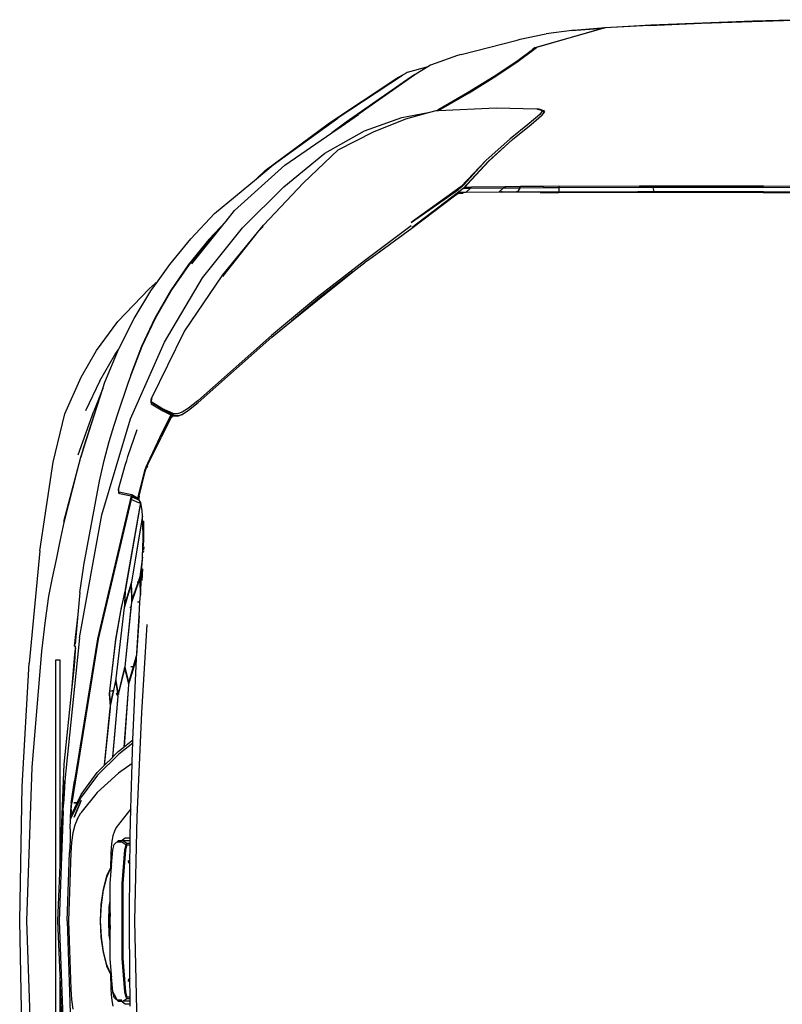
# Model space of a CAD drawing. Units: inches. Extents: x 22042254 to 25404563, y 17568978 to 17626777.
# Tile 3 of 45: x 22042254.0718 to 22042254.5426, y 17568978.1657 to 17568978.7735. Entities that reach past the tile are written whole.
import ezdxf

# ---------------------------------------------------------------- set-up
doc = ezdxf.new("R2010")
doc.units = ezdxf.units.IN
doc.header["$MEASUREMENT"] = 0
doc.layers.add('A-SITE-VEHI', color=8, linetype='Continuous', lineweight=18)
doc.layers.add('Edges', color=250, linetype='Continuous')

# ---------------------------------------------------------------- blocks, each defined once
blk = doc.blocks.new('Nissan Qashqai pl')
at = {"layer": 'Edges'}
for p, q in [((7.32157, 11.66208), (7.32157, 12.18208)), ((7.32607, 12.18208), (7.32607, 11.97794)), ((7.29801, 12.07497), (7.29279, 11.92208)), ((7.33017, 12.07853), (7.32607, 11.97794)), ((7.28835, 12.05625), (7.28572, 11.92208)), ((7.32507, 11.92208), (7.32911, 12.03155)), ((7.40018, 11.92208), (7.40245, 12.02601)), ((7.33294, 11.92208), (7.33653, 12.02372)), ((7.33733, 12.00038), (7.33865, 12.00996)), ((7.37751, 12.0015), (7.37864, 12.00699)), ((7.39589, 12.00706), (7.39588, 12.00508)), ((7.33667, 11.99003), (7.33733, 12.00038)), ((7.37683, 11.99537), (7.37751, 12.0015)), ((7.37985, 11.99831), (7.3787, 11.99283)), ((7.38081, 11.99933), (7.37985, 11.99831)), ((7.38074, 11.99908), (7.37985, 11.99831)), ((7.38002, 11.99534), (7.38305, 12.00106)), ((7.38074, 11.99908), (7.38081, 11.99933)), ((7.38104, 11.99933), (7.38074, 11.99908)), ((7.38081, 11.99933), (7.38402, 12.00208)), ((7.38104, 11.99933), (7.38081, 11.99933)), ((7.38305, 12.00106), (7.38104, 11.99933)), ((7.38659, 12.00106), (7.38305, 12.00106)), ((7.38402, 12.00208), (7.38696, 12.00208)), ((7.38683, 12.00198), (7.38659, 12.00106)), ((7.3875, 12.00106), (7.38659, 12.00106)), ((7.38696, 12.00208), (7.38683, 12.00198)), ((7.39094, 12.00508), (7.38696, 12.00208)), ((7.38696, 12.00208), (7.38847, 12.00208)), ((7.38847, 12.00208), (7.39254, 11.99933)), ((7.39551, 12.00208), (7.38847, 12.00208)), ((7.39041, 11.99283), (7.39156, 11.99831)), ((7.39564, 12.00508), (7.39094, 12.00508)), ((7.39288, 11.99808), (7.39173, 11.99259)), ((7.39254, 11.99933), (7.39582, 11.99933)), ((7.39254, 11.99933), (7.39288, 11.99808)), ((7.3958, 11.99808), (7.39288, 11.99808)), ((7.39551, 12.00208), (7.39584, 12.00183)), ((7.39588, 12.0049), (7.39564, 12.00508)), ((7.39588, 12.00508), (7.39564, 12.00508)), ((7.3958, 11.99808), (7.39564, 11.98012)), ((7.39582, 11.99933), (7.3958, 11.99808)), ((7.39584, 12.00183), (7.39582, 11.99933)), ((7.39588, 12.0049), (7.39584, 12.00183)), ((7.39588, 12.00508), (7.39588, 12.0049)), ((7.33429, 11.92208), (7.33667, 11.99003)), ((7.37614, 11.97511), (7.37648, 11.98901)), ((7.37648, 11.98901), (7.37683, 11.99537)), ((7.3787, 11.99283), (7.37743, 11.97775)), ((7.3787, 11.99283), (7.38002, 11.99534)), ((7.38759, 11.95948), (7.39041, 11.99283)), ((7.39173, 11.99259), (7.38892, 11.95935)), ((7.32607, 11.9764), (7.32607, 11.97794)), ((7.37614, 11.97511), (7.37686, 11.97673)), ((7.37686, 11.97673), (7.3771, 11.97702)), ((7.37713, 11.97709), (7.3771, 11.97702)), ((7.37743, 11.97775), (7.37713, 11.97709)), ((7.37713, 11.97709), (7.3774, 11.97738)), ((7.3774, 11.97738), (7.37727, 11.97594)), ((7.3774, 11.97738), (7.37743, 11.97775)), ((7.39385, 11.98229), (7.39564, 11.98012)), ((7.39563, 11.97885), (7.39385, 11.981)), ((7.39563, 11.97885), (7.3951, 11.92208)), ((7.39564, 11.98012), (7.39563, 11.97885)), ((7.32607, 11.9764), (7.3238, 11.92208)), ((7.37239, 11.9667), (7.37614, 11.97511)), ((7.37707, 11.97569), (7.37268, 11.96585)), ((7.37727, 11.97594), (7.37588, 11.95948)), ((7.37727, 11.97594), (7.37707, 11.97569)), ((7.36896, 11.95363), (7.37239, 11.9667)), ((7.37268, 11.96585), (7.36932, 11.95303)), ((7.37588, 11.95948), (7.37588, 11.94171)), ((7.38759, 11.88468), (7.38759, 11.95948)), ((7.38892, 11.95935), (7.38892, 11.88481)), ((7.36681, 11.93841), (7.36896, 11.95363)), ((7.36932, 11.95303), (7.3672, 11.9381)), ((7.36607, 11.92208), (7.36681, 11.93841)), ((7.3672, 11.9381), (7.36648, 11.92208)), ((7.37588, 11.94171), (7.37512, 11.93632)), ((7.37588, 11.94171), (7.37588, 11.93029)), ((7.37512, 11.93632), (7.37448, 11.92208)), ((7.37551, 11.92208), (7.37588, 11.93029)), ((7.37588, 11.93029), (7.37588, 11.91388)), ((7.28572, 11.92208), (7.28835, 11.78791)), ((7.29279, 11.92208), (7.29801, 11.76919)), ((7.3238, 11.92208), (7.32607, 11.86622)), ((7.32911, 11.81261), (7.32507, 11.92208)), ((7.33294, 11.92208), (7.33535, 11.85392)), ((7.33667, 11.85414), (7.33429, 11.92208)), ((7.36681, 11.90575), (7.36607, 11.92208)), ((7.36648, 11.92208), (7.3672, 11.90606)), ((7.37448, 11.92208), (7.37512, 11.90785)), ((7.37588, 11.91388), (7.37551, 11.92208)), ((7.3951, 11.92208), (7.39563, 11.86531)), ((7.40245, 11.81815), (7.40018, 11.92208)), ((7.37588, 11.91388), (7.37588, 11.90246)), ((7.36896, 11.89053), (7.36681, 11.90575)), ((7.3672, 11.90606), (7.36932, 11.89113)), ((7.37512, 11.90785), (7.37588, 11.90246)), ((7.37588, 11.90246), (7.37588, 11.88468)), ((7.37239, 11.87746), (7.36896, 11.89053)), ((7.36932, 11.89113), (7.37268, 11.87831)), ((7.37588, 11.88468), (7.37727, 11.86822)), ((7.39041, 11.85133), (7.38759, 11.88468)), ((7.38892, 11.88481), (7.39173, 11.85157)), ((7.37614, 11.86905), (7.37239, 11.87746)), ((7.37268, 11.87831), (7.37707, 11.86848)), ((7.37648, 11.85515), (7.37614, 11.86905)), ((7.37686, 11.86743), (7.37614, 11.86905)), ((7.32607, 11.86622), (7.33017, 11.76563)), ((7.32607, 11.86622), (7.32607, 11.66208)), ((7.3771, 11.86714), (7.37686, 11.86743)), ((7.37707, 11.86848), (7.37727, 11.86822)), ((7.3771, 11.86714), (7.37713, 11.86707)), ((7.37713, 11.86707), (7.37743, 11.86641)), ((7.3774, 11.86678), (7.37713, 11.86707)), ((7.37727, 11.86822), (7.3774, 11.86678)), ((7.3774, 11.86678), (7.37743, 11.86641)), ((7.37743, 11.86641), (7.3787, 11.85133)), ((7.39385, 11.86316), (7.39563, 11.86531)), ((7.39564, 11.86404), (7.39385, 11.86187)), ((7.39563, 11.86531), (7.39564, 11.86404)), ((7.39564, 11.86404), (7.3958, 11.84608)), ((7.33608, 11.84164), (7.33535, 11.85392)), ((7.33733, 11.84378), (7.33667, 11.85414)), ((7.37683, 11.8488), (7.37648, 11.85515)), ((7.3787, 11.85133), (7.37985, 11.84585)), ((7.39156, 11.84585), (7.39041, 11.85133)), ((7.39173, 11.85157), (7.39288, 11.84608)), ((7.33619, 11.83012), (7.33608, 11.84164)), ((7.33865, 11.8342), (7.33733, 11.84378)), ((7.37751, 11.84267), (7.37683, 11.8488)), ((7.37864, 11.83717), (7.37751, 11.84267)), ((7.37985, 11.84585), (7.38081, 11.84483)), ((7.38081, 11.84483), (7.38074, 11.84508)), ((7.38081, 11.84483), (7.38104, 11.84483)), ((7.38402, 11.84208), (7.38081, 11.84483)), ((7.38305, 11.8431), (7.3875, 11.8431)), ((7.38696, 11.84208), (7.38402, 11.84208)), ((7.38696, 11.84208), (7.39094, 11.83908)), ((7.38847, 11.84208), (7.38696, 11.84208)), ((7.3875, 11.8431), (7.39156, 11.84585)), ((7.39254, 11.84483), (7.38847, 11.84208)), ((7.39551, 11.84208), (7.38847, 11.84208)), ((7.39288, 11.84608), (7.39254, 11.84483)), ((7.39582, 11.84483), (7.39254, 11.84483)), ((7.39288, 11.84608), (7.3958, 11.84608)), ((7.39584, 11.84233), (7.39551, 11.84208)), ((7.39564, 11.83908), (7.39587, 11.83925)), ((7.3958, 11.84608), (7.39582, 11.84483)), ((7.39582, 11.84483), (7.39584, 11.84233)), ((7.39584, 11.84233), (7.39587, 11.83925)), ((7.39587, 11.83925), (7.39587, 11.83908)), ((7.33619, 11.83012), (7.33653, 11.82044)), ((7.3407, 11.82658), (7.33865, 11.8342)), ((7.38014, 11.8327), (7.37864, 11.83717)), ((7.38184, 11.82907), (7.38014, 11.8327)), ((7.39094, 11.83908), (7.39564, 11.83908)), ((7.39564, 11.83908), (7.39587, 11.83908)), ((7.39587, 11.83908), (7.39589, 11.8371)), ((7.39589, 11.8371), (7.3966, 11.81032)), ((7.33615, 11.81939), (7.33653, 11.82044)), ((7.33672, 11.81955), (7.33615, 11.81939)), ((7.33653, 11.82044), (7.34711, 11.79873)), ((7.34316, 11.82104), (7.3407, 11.82658)), ((7.34316, 11.82104), (7.34679, 11.81424)), ((7.3966, 11.81032), (7.38184, 11.82907)), ((7.32911, 11.81261), (7.32941, 11.80569)), ((7.33645, 11.81201), (7.33615, 11.81939)), ((7.33691, 11.80472), (7.33645, 11.81201)), ((7.33686, 11.81546), (7.33737, 11.81653)), ((7.33691, 11.81132), (7.33686, 11.81546)), ((7.33686, 11.81546), (7.33805, 11.81508)), ((7.33691, 11.81132), (7.33767, 11.80437)), ((7.33737, 11.81653), (7.33805, 11.81508)), ((7.33805, 11.81508), (7.34299, 11.80448)), ((7.34013, 11.81856), (7.34308, 11.8112)), ((7.347, 11.80211), (7.34013, 11.81856)), ((7.34308, 11.8112), (7.347, 11.80211)), ((7.36303, 11.79404), (7.34679, 11.81424)), ((7.3966, 11.81032), (7.39782, 11.76508)), ((7.40723, 11.71423), (7.40245, 11.81815)), ((7.33008, 11.79493), (7.32941, 11.80569)), ((7.3295, 11.80119), (7.33087, 11.78224)), ((7.3295, 11.80119), (7.33008, 11.79493)), ((7.33691, 11.80472), (7.34048, 11.78254)), ((7.33771, 11.80416), (7.33767, 11.80437)), ((7.34104, 11.78371), (7.33771, 11.80416)), ((7.34299, 11.80448), (7.33961, 11.8043)), ((7.33961, 11.8043), (7.34314, 11.80416)), ((7.34299, 11.80448), (7.34314, 11.80416)), ((7.34314, 11.80416), (7.34693, 11.79606)), ((7.33087, 11.78224), (7.33008, 11.79493)), ((7.34693, 11.79606), (7.36309, 11.77403)), ((7.36331, 11.77672), (7.34711, 11.79873)), ((7.38423, 11.77487), (7.36303, 11.79404)), ((7.28835, 11.78791), (7.29513, 11.66508)), ((7.33168, 11.77242), (7.33087, 11.78224)), ((7.36347, 11.6409), (7.34048, 11.78254)), ((7.34263, 11.77348), (7.34104, 11.78371)), ((7.34554, 11.63996), (7.33168, 11.77242)), ((7.36397, 11.64129), (7.34263, 11.77348)), ((7.36309, 11.77403), (7.37008, 11.76708)), ((7.38449, 11.75584), (7.36331, 11.77672)), ((7.39782, 11.76508), (7.38423, 11.77487)), ((7.29801, 11.76919), (7.30777, 11.65317)), ((7.33017, 11.76563), (7.33778, 11.69209)), ((7.37589, 11.71006), (7.37008, 11.76708)), ((7.37008, 11.76708), (7.37036, 11.76681)), ((7.37036, 11.76681), (7.37608, 11.71004)), ((7.37036, 11.76681), (7.37826, 11.75896)), ((7.39782, 11.76508), (7.39816, 11.75211)), ((7.38357, 11.6983), (7.37826, 11.75896)), ((7.37826, 11.75896), (7.37876, 11.75846)), ((7.37876, 11.75846), (7.38403, 11.69824)), ((7.37876, 11.75846), (7.38409, 11.75317)), ((7.38409, 11.75317), (7.38964, 11.74878)), ((7.39848, 11.74482), (7.38449, 11.75584)), ((7.39816, 11.75211), (7.39848, 11.74482)), ((7.39414, 11.68653), (7.38964, 11.74878)), ((7.38964, 11.74878), (7.39027, 11.74828)), ((7.39027, 11.74828), (7.39449, 11.68648)), ((7.39027, 11.74828), (7.39862, 11.74167)), ((7.39848, 11.74482), (7.39862, 11.74167)), ((7.39862, 11.74167), (7.40182, 11.66777)), ((7.41241, 11.62655), (7.40723, 11.71423)), ((7.37498, 11.69572), (7.37596, 11.70814)), ((7.37623, 11.70617), (7.37575, 11.69593)), ((7.37596, 11.70814), (7.37589, 11.71006)), ((7.37608, 11.71004), (7.37634, 11.7081)), ((7.37623, 11.70617), (7.37642, 11.70614)), ((7.37634, 11.7081), (7.38127, 11.68424)), ((7.37642, 11.70614), (7.37916, 11.6924)), ((7.33778, 11.69209), (7.34072, 11.65629)), ((7.33778, 11.69209), (7.33996, 11.67104)), ((7.38128, 11.64204), (7.37498, 11.69572)), ((7.37575, 11.69593), (7.37562, 11.69326)), ((7.37916, 11.6924), (7.37562, 11.69326)), ((7.37562, 11.69326), (7.38154, 11.64126)), ((7.37568, 11.69592), (7.37575, 11.69593)), ((7.38118, 11.68226), (7.37916, 11.6924)), ((7.38174, 11.68442), (7.38322, 11.69486)), ((7.38379, 11.69443), (7.38202, 11.68226)), ((7.38243, 11.69547), (7.38357, 11.6983)), ((7.3835, 11.69733), (7.38243, 11.69547)), ((7.38336, 11.69586), (7.38243, 11.69547)), ((7.38243, 11.69547), (7.38322, 11.69486)), ((7.38324, 11.69498), (7.38243, 11.69547)), ((7.38322, 11.69486), (7.38379, 11.69443)), ((7.38324, 11.69498), (7.38336, 11.69586)), ((7.38377, 11.69466), (7.38324, 11.69498)), ((7.3837, 11.696), (7.38336, 11.69586)), ((7.3835, 11.69733), (7.38357, 11.6983)), ((7.38361, 11.69752), (7.3835, 11.69733)), ((7.38361, 11.69752), (7.38357, 11.6983)), ((7.38403, 11.69824), (7.38361, 11.69752)), ((7.38438, 11.69629), (7.3837, 11.696)), ((7.38377, 11.69466), (7.3837, 11.696)), ((7.38426, 11.69437), (7.38377, 11.69466)), ((7.38429, 11.69425), (7.38379, 11.69443)), ((7.38426, 11.69437), (7.38438, 11.69629)), ((7.38429, 11.69425), (7.38426, 11.69437)), ((7.38773, 11.68027), (7.38429, 11.69425)), ((7.38438, 11.69629), (7.39028, 11.67251)), ((7.38152, 11.68035), (7.38118, 11.68226)), ((7.38127, 11.68424), (7.38174, 11.68442)), ((7.3817, 11.68412), (7.38127, 11.68424)), ((7.3817, 11.68412), (7.38174, 11.68442)), ((7.38202, 11.68226), (7.38195, 11.68031)), ((7.39093, 11.67275), (7.39387, 11.6846)), ((7.39425, 11.68274), (7.39127, 11.6705)), ((7.39387, 11.6846), (7.39414, 11.68653)), ((7.39425, 11.68274), (7.39494, 11.68257)), ((7.39425, 11.68274), (7.39497, 11.68247)), ((7.39449, 11.68648), (7.39509, 11.68353)), ((7.39497, 11.68247), (7.39494, 11.68257)), ((7.39898, 11.66858), (7.39497, 11.68247)), ((7.39509, 11.68353), (7.40207, 11.66087)), ((7.38995, 11.60941), (7.38152, 11.68035)), ((7.38195, 11.68031), (7.39032, 11.60945)), ((7.38737, 11.68027), (7.38773, 11.68027)), ((7.39008, 11.67074), (7.38773, 11.68027)), ((7.39093, 11.67275), (7.39028, 11.67251)), ((7.39087, 11.67252), (7.39028, 11.67251)), ((7.39087, 11.67252), (7.39093, 11.67275)), ((7.3059, 11.55319), (7.29513, 11.66508)), ((7.33996, 11.67104), (7.34097, 11.65941)), ((7.39046, 11.66873), (7.39008, 11.67074)), ((7.3966, 11.6095), (7.39046, 11.66873)), ((7.39127, 11.6705), (7.39107, 11.66865)), ((7.39107, 11.66865), (7.39768, 11.60417)), ((7.39898, 11.66858), (7.39666, 11.66858)), ((7.4017, 11.65916), (7.39898, 11.66858)), ((7.40182, 11.66777), (7.40224, 11.66093)), ((7.30777, 11.65317), (7.31133, 11.62243)), ((7.32607, 11.66208), (7.32157, 11.66208)), ((7.34072, 11.65629), (7.34131, 11.65087)), ((7.34097, 11.65941), (7.34133, 11.65108)), ((7.40216, 11.65713), (7.4017, 11.65916)), ((7.40224, 11.66093), (7.40207, 11.66087)), ((7.40224, 11.66086), (7.40207, 11.66087)), ((7.40484, 11.618), (7.40216, 11.65713)), ((7.40224, 11.66093), (7.40224, 11.66086)), ((7.40224, 11.66086), (7.40484, 11.618)), ((7.34009, 11.64801), (7.34004, 11.64799)), ((7.3438, 11.61665), (7.34004, 11.64799)), ((7.34097, 11.64796), (7.34009, 11.64801)), ((7.34097, 11.64796), (7.34131, 11.65087)), ((7.34097, 11.64796), (7.34145, 11.64799)), ((7.34144, 11.64796), (7.34097, 11.64796)), ((7.3438, 11.61665), (7.34121, 11.64598)), ((7.34133, 11.65108), (7.34131, 11.65087)), ((7.34131, 11.65087), (7.34154, 11.6488)), ((7.34554, 11.63996), (7.36761, 11.51724)), ((7.39705, 11.49808), (7.36347, 11.6409)), ((7.39678, 11.50175), (7.36397, 11.64129)), ((7.3869, 11.60943), (7.38128, 11.64204)), ((7.38154, 11.64126), (7.38644, 11.61311)), ((7.31133, 11.62243), (7.31494, 11.59842)), ((7.34574, 11.59466), (7.3438, 11.61665)), ((7.40484, 11.618), (7.40567, 11.60418)), ((7.38644, 11.61311), (7.39089, 11.59332)), ((7.39116, 11.59143), (7.3869, 11.60943)), ((7.39012, 11.60735), (7.38995, 11.60941)), ((7.39099, 11.59348), (7.39012, 11.60735)), ((7.39032, 11.60945), (7.3908, 11.60755)), ((7.39058, 11.60552), (7.39095, 11.60545)), ((7.39058, 11.60552), (7.39098, 11.60538)), ((7.39058, 11.60552), (7.39141, 11.59144)), ((7.3908, 11.60755), (7.39654, 11.58812)), ((7.39098, 11.60538), (7.39095, 11.60545)), ((7.39668, 11.58624), (7.39098, 11.60538)), ((7.3966, 11.6095), (7.39566, 11.6095)), ((7.39715, 11.60416), (7.3966, 11.6095)), ((7.39722, 11.60211), (7.39715, 11.60416)), ((7.39768, 11.60417), (7.39823, 11.60225)), ((7.40567, 11.60418), (7.40319, 11.60418)), ((7.40567, 11.60418), (7.40611, 11.59696)), ((7.31494, 11.59842), (7.3186, 11.58002)), ((7.34574, 11.59466), (7.34938, 11.57004)), ((7.39684, 11.58823), (7.39722, 11.60211)), ((7.39774, 11.60029), (7.39733, 11.58621)), ((7.39774, 11.60029), (7.39827, 11.60018)), ((7.39774, 11.60029), (7.39831, 11.60008)), ((7.39823, 11.60225), (7.40485, 11.58292)), ((7.39831, 11.60008), (7.39827, 11.60018)), ((7.40376, 11.5843), (7.39831, 11.60008)), ((7.40533, 11.58312), (7.40611, 11.59688)), ((7.40611, 11.59688), (7.40611, 11.59696)), ((7.40611, 11.59688), (7.40642, 11.59185)), ((7.39099, 11.59348), (7.39089, 11.59332)), ((7.39101, 11.59337), (7.39089, 11.59332)), ((7.39156, 11.58943), (7.39116, 11.59143)), ((7.39141, 11.59144), (7.39169, 11.5895)), ((7.40622, 11.5053), (7.39156, 11.58943)), ((7.39169, 11.5895), (7.40648, 11.50498)), ((7.39684, 11.58823), (7.39654, 11.58812)), ((7.39714, 11.58424), (7.39668, 11.58624)), ((7.39684, 11.58823), (7.39731, 11.58844)), ((7.40828, 11.51835), (7.39714, 11.58424)), ((7.39733, 11.58621), (7.39747, 11.58427)), ((7.39747, 11.58427), (7.40836, 11.51976)), ((7.40376, 11.5843), (7.40279, 11.5843)), ((7.40488, 11.58107), (7.40376, 11.5843)), ((7.40642, 11.59185), (7.40597, 11.58338)), ((7.40642, 11.59185), (7.40687, 11.58436)), ((7.40687, 11.58436), (7.40791, 11.56437)), ((7.3186, 11.58002), (7.32232, 11.56164)), ((7.40533, 11.58312), (7.40485, 11.58292)), ((7.40532, 11.58299), (7.40485, 11.58292)), ((7.40539, 11.57906), (7.40488, 11.58107)), ((7.40597, 11.58327), (7.40532, 11.58299)), ((7.40532, 11.58299), (7.40533, 11.58312)), ((7.40597, 11.58338), (7.40533, 11.58312)), ((7.40814, 11.55935), (7.40539, 11.57906)), ((7.40597, 11.58327), (7.40585, 11.58097)), ((7.40585, 11.58097), (7.40588, 11.57905)), ((7.40588, 11.57905), (7.40791, 11.56437)), ((7.40597, 11.58338), (7.40597, 11.58327)), ((7.40813, 11.57111), (7.40752, 11.58276)), ((7.34938, 11.57004), (7.3497, 11.56742)), ((7.34938, 11.57004), (7.34978, 11.56736)), ((7.3497, 11.56742), (7.36534, 11.48377)), ((7.40791, 11.56437), (7.40811, 11.56038)), ((7.40791, 11.56437), (7.40812, 11.56285)), ((7.32232, 11.56164), (7.3261, 11.54328)), ((7.40811, 11.56038), (7.40814, 11.55935)), ((7.40814, 11.55935), (7.40871, 11.54047)), ((7.40926, 11.55458), (7.40949, 11.55292)), ((7.3059, 11.55319), (7.31925, 11.46451)), ((7.40923, 11.54161), (7.40902, 11.54853)), ((7.4096, 11.54898), (7.40916, 11.55209)), ((7.3261, 11.54328), (7.32996, 11.52493)), ((7.40871, 11.54047), (7.40865, 11.52464)), ((7.40921, 11.52579), (7.40923, 11.54161)), ((7.40908, 11.52353), (7.40921, 11.52579)), ((7.3297, 11.52373), (7.34671, 11.45961)), ((7.32996, 11.52493), (7.34671, 11.45961)), ((7.36761, 11.51724), (7.39627, 11.42146)), ((7.40828, 11.51835), (7.40795, 11.51289)), ((7.40836, 11.51976), (7.40828, 11.51835)), ((7.40865, 11.52464), (7.40836, 11.51976)), ((7.40795, 11.51289), (7.4066, 11.50521)), ((7.38529, 11.49584), (7.38412, 11.49562)), ((7.38437, 11.49158), (7.38412, 11.49562)), ((7.39764, 11.49714), (7.38458, 11.49463)), ((7.38529, 11.49584), (7.38458, 11.49463)), ((7.38529, 11.49584), (7.39705, 11.49808)), ((7.40464, 11.5053), (7.39678, 11.50175)), ((7.39804, 11.49925), (7.39678, 11.50175)), ((7.39705, 11.49808), (7.39833, 11.49833)), ((7.40264, 11.50022), (7.39764, 11.49714)), ((7.39804, 11.49925), (7.40478, 11.50242)), ((7.4012, 11.50009), (7.39804, 11.49925)), ((7.39833, 11.49833), (7.4012, 11.50009)), ((7.4012, 11.50009), (7.40335, 11.50141)), ((7.40299, 11.50047), (7.40264, 11.50022)), ((7.40299, 11.50047), (7.40276, 11.50042)), ((7.40326, 11.50066), (7.40299, 11.50047)), ((7.40417, 11.50199), (7.40326, 11.50066)), ((7.4033, 11.50053), (7.40326, 11.50066)), ((7.40335, 11.50054), (7.4033, 11.50053)), ((7.41007, 11.47333), (7.4033, 11.50053)), ((7.40335, 11.50141), (7.40417, 11.50199)), ((7.40425, 11.50164), (7.40405, 11.50122)), ((7.40431, 11.5014), (7.40405, 11.50122)), ((7.40405, 11.50122), (7.41077, 11.47382)), ((7.40417, 11.50199), (7.40443, 11.50199)), ((7.40425, 11.50164), (7.40417, 11.50199)), ((7.40443, 11.50199), (7.40425, 11.50164)), ((7.40431, 11.5014), (7.40425, 11.50164)), ((7.40461, 11.50161), (7.40431, 11.5014)), ((7.40447, 11.50076), (7.40431, 11.5014)), ((7.40456, 11.50227), (7.40443, 11.50199)), ((7.40443, 11.50199), (7.40463, 11.50199)), ((7.4048, 11.50082), (7.40447, 11.50076)), ((7.40502, 11.49854), (7.40447, 11.50076)), ((7.40456, 11.50227), (7.40478, 11.50242)), ((7.40497, 11.50227), (7.40456, 11.50227)), ((7.40456, 11.50227), (7.40463, 11.50199)), ((7.40469, 11.50176), (7.40461, 11.50161)), ((7.40463, 11.50199), (7.40469, 11.50176)), ((7.40463, 11.50199), (7.40482, 11.50199)), ((7.40622, 11.5053), (7.40464, 11.5053)), ((7.40482, 11.50199), (7.40469, 11.50176)), ((7.40478, 11.50242), (7.40523, 11.50274)), ((7.40515, 11.5026), (7.40478, 11.50242)), ((7.40497, 11.50227), (7.40482, 11.50199)), ((7.40515, 11.5026), (7.40497, 11.50227)), ((7.40523, 11.50274), (7.40515, 11.5026)), ((7.40632, 11.5047), (7.40523, 11.50274)), ((7.40632, 11.5047), (7.40622, 11.5053)), ((7.40648, 11.50498), (7.40632, 11.5047)), ((7.4066, 11.50521), (7.40648, 11.50498)), ((7.38458, 11.49463), (7.38437, 11.49158)), ((7.38437, 11.49158), (7.39136, 11.46669)), ((7.36534, 11.48377), (7.36995, 11.46286)), ((7.39136, 11.46669), (7.39248, 11.46286)), ((7.41147, 11.46951), (7.41007, 11.47333)), ((7.41077, 11.47382), (7.41219, 11.47)), ((7.41315, 11.46587), (7.41147, 11.46951)), ((7.41219, 11.47), (7.41393, 11.46637)), ((7.41256, 11.46999), (7.41248, 11.47021)), ((7.41324, 11.46853), (7.41256, 11.46999)), ((7.41393, 11.46637), (7.42672, 11.44006)), ((7.31925, 11.46451), (7.3309, 11.41659)), ((7.34401, 11.45722), (7.35959, 11.41392)), ((7.34891, 11.45171), (7.34671, 11.45961)), ((7.34671, 11.45961), (7.36864, 11.39135)), ((7.36995, 11.46286), (7.375, 11.44419)), ((7.39248, 11.46286), (7.39374, 11.45905)), ((7.39374, 11.45905), (7.40289, 11.43211)), ((7.42553, 11.43981), (7.41315, 11.46587)), ((7.34891, 11.45171), (7.36864, 11.39135)), ((7.375, 11.44419), (7.37986, 11.42777)), ((7.42553, 11.43981), (7.43673, 11.41738)), ((7.43787, 11.41791), (7.42672, 11.44006)), ((7.37986, 11.42777), (7.38454, 11.41358)), ((7.39627, 11.42146), (7.43015, 11.3449)), ((7.43587, 11.41698), (7.43673, 11.41738)), ((7.43832, 11.417), (7.43673, 11.41738)), ((7.43751, 11.42004), (7.43844, 11.41817)), ((7.43787, 11.41791), (7.43844, 11.41817)), ((7.4389, 11.41727), (7.43787, 11.41791)), ((7.43832, 11.417), (7.43787, 11.41791)), ((7.4389, 11.41727), (7.43832, 11.417)), ((7.43844, 11.41817), (7.43873, 11.41831)), ((7.43873, 11.41831), (7.44298, 11.41881)), ((7.4389, 11.41727), (7.44004, 11.41781)), ((7.44418, 11.41831), (7.44004, 11.41781)), ((7.44298, 11.41881), (7.44771, 11.41717)), ((7.44771, 11.41717), (7.44418, 11.41831)), ((7.44771, 11.41717), (7.45415, 11.41285)), ((7.3309, 11.41659), (7.34698, 11.37976)), ((7.36552, 11.38372), (7.3514, 11.41334)), ((7.36864, 11.39135), (7.35959, 11.41392)), ((7.38454, 11.41358), (7.39247, 11.38995)), ((7.42821, 11.41133), (7.41689, 11.40438)), ((7.41697, 11.40649), (7.42833, 11.41346)), ((7.42961, 11.41292), (7.4183, 11.40596)), ((7.43873, 11.41619), (7.42821, 11.41133)), ((7.42833, 11.41346), (7.43587, 11.41698)), ((7.42961, 11.41292), (7.43832, 11.417)), ((7.44309, 11.41655), (7.43873, 11.41619)), ((7.44789, 11.41487), (7.44309, 11.41655)), ((7.4541, 11.41081), (7.44789, 11.41487)), ((7.46355, 11.40337), (7.4541, 11.41081)), ((7.45415, 11.41285), (7.46382, 11.40513)), ((7.41665, 11.40488), (7.41697, 11.40649)), ((7.41716, 11.40469), (7.41665, 11.40488)), ((7.41687, 11.40359), (7.41665, 11.40488)), ((7.41687, 11.40359), (7.41686, 11.40296)), ((7.41686, 11.40296), (7.41723, 11.40107)), ((7.41689, 11.40438), (7.41687, 11.40359)), ((7.41717, 11.40184), (7.41687, 11.40359)), ((7.41716, 11.40469), (7.41689, 11.40438)), ((7.4183, 11.40596), (7.41716, 11.40469)), ((7.41744, 11.4013), (7.41717, 11.40184)), ((7.41723, 11.40107), (7.44978, 11.33488)), ((7.41744, 11.4013), (7.41747, 11.40124)), ((7.53689, 11.33848), (7.46355, 11.40337)), ((7.46382, 11.40513), (7.53708, 11.33997)), ((7.36864, 11.39135), (7.37074, 11.38491)), ((7.39247, 11.38995), (7.39379, 11.3859)), ((7.34698, 11.37976), (7.36237, 11.35349)), ((7.36552, 11.38372), (7.38053, 11.35758)), ((7.37074, 11.38491), (7.38426, 11.35219)), ((7.39379, 11.3859), (7.39513, 11.38217)), ((7.39513, 11.38217), (7.39648, 11.37869)), ((7.39621, 11.37814), (7.39648, 11.37869)), ((7.40715, 11.34933), (7.39621, 11.37814)), ((7.39648, 11.37869), (7.39687, 11.3777)), ((7.39687, 11.3777), (7.40781, 11.34902)), ((7.36237, 11.35349), (7.38367, 11.32447)), ((7.38053, 11.35758), (7.38426, 11.35219)), ((7.38426, 11.35219), (7.38446, 11.35171)), ((7.38446, 11.35171), (7.39973, 11.32146)), ((7.42053, 11.32124), (7.40715, 11.34933)), ((7.40781, 11.34902), (7.42115, 11.32101)), ((7.43015, 11.3449), (7.46788, 11.28072)), ((7.58274, 11.30006), (7.53689, 11.33848)), ((7.53708, 11.33997), (7.55684, 11.32404)), ((7.44978, 11.33488), (7.48836, 11.27781)), ((7.38367, 11.32447), (7.41469, 11.29179)), ((7.39973, 11.32146), (7.41661, 11.29389)), ((7.43626, 11.29398), (7.42053, 11.32124)), ((7.42115, 11.32101), (7.4369, 11.29377)), ((7.58398, 11.30127), (7.55684, 11.32404)), ((7.55684, 11.32404), (7.58288, 11.30303)), ((7.6296, 11.2639), (7.58274, 11.30006)), ((7.58288, 11.30303), (7.61803, 11.27504)), ((7.61803, 11.27504), (7.58398, 11.30127)), ((7.41469, 11.29179), (7.42386, 11.28371)), ((7.41661, 11.29389), (7.42386, 11.28371)), ((7.45423, 11.26769), (7.43626, 11.29398)), ((7.4369, 11.29377), (7.45491, 11.26748)), ((7.42386, 11.28371), (7.4354, 11.26752)), ((7.46788, 11.28072), (7.50805, 11.2311)), ((7.48817, 11.27966), (7.52431, 11.23409)), ((7.48836, 11.27781), (7.52891, 11.22832)), ((7.61803, 11.27504), (7.63007, 11.26544)), ((7.4354, 11.26752), (7.45654, 11.24186)), ((7.47438, 11.24268), (7.45423, 11.26769)), ((7.45491, 11.26748), (7.47504, 11.24255)), ((7.45735, 11.26699), (7.48846, 11.22834)), ((7.67598, 11.22893), (7.6296, 11.2639)), ((7.63007, 11.26544), (7.63056, 11.26506)), ((7.63056, 11.26506), (7.63059, 11.26504)), ((7.63059, 11.26504), (7.6373, 11.26013)), ((7.6373, 11.26013), (7.67691, 11.23122)), ((7.45654, 11.24186), (7.48015, 11.2168)), ((7.49177, 11.22424), (7.47438, 11.24268)), ((7.47504, 11.24255), (7.47703, 11.24044)), ((7.47703, 11.24044), (7.47653, 11.24106)), ((7.47703, 11.24053), (7.47751, 11.23993)), ((7.47838, 11.23878), (7.47703, 11.24044)), ((7.47703, 11.24044), (7.47751, 11.23993)), ((7.47751, 11.23993), (7.47871, 11.23847)), ((7.47751, 11.23993), (7.47869, 11.23868)), ((7.47869, 11.23868), (7.47824, 11.23925)), ((7.4795, 11.2377), (7.47869, 11.23868)), ((7.47869, 11.23868), (7.48846, 11.22834)), ((7.50805, 11.2311), (7.5492, 11.19016)), ((7.52431, 11.23409), (7.52857, 11.22958)), ((7.67691, 11.23122), (7.71943, 11.19922)), ((7.72318, 11.19554), (7.67713, 11.2307)), ((7.48846, 11.22834), (7.49177, 11.22424)), ((7.49177, 11.22424), (7.50008, 11.21391)), ((7.52891, 11.22832), (7.56866, 11.18624)), ((7.72614, 11.18985), (7.67617, 11.22557)), ((7.67617, 11.22557), (7.72327, 11.1928)), ((7.48015, 11.2168), (7.52174, 11.18228)), ((7.50008, 11.21391), (7.55011, 11.16843)), ((7.71943, 11.19922), (7.72318, 11.19658)), ((7.72318, 11.19658), (7.72785, 11.19647)), ((7.72807, 11.19181), (7.72318, 11.19554)), ((7.72318, 11.19554), (7.72455, 11.19553)), ((7.72667, 11.19023), (7.72327, 11.1928)), ((7.72467, 11.19542), (7.72455, 11.19553)), ((7.72455, 11.19553), (7.72942, 11.19548)), ((7.72807, 11.19181), (7.72986, 11.19044)), ((7.73491, 11.19175), (7.72807, 11.19181)), ((7.75301, 11.16475), (7.72807, 11.19181)), ((7.72942, 11.19548), (7.73096, 11.19549)), ((7.73096, 11.19549), (7.73491, 11.19175)), ((7.73096, 11.19549), (7.76399, 11.19528)), ((7.76799, 11.19147), (7.73491, 11.19175)), ((7.76399, 11.19528), (7.7636, 11.19566)), ((7.76799, 11.19147), (7.76399, 11.19528)), ((7.76399, 11.19528), (7.76622, 11.19527)), ((7.76586, 11.19567), (7.76622, 11.19527)), ((7.76622, 11.19527), (7.76683, 11.19458)), ((7.76622, 11.19527), (7.78115, 11.19519)), ((7.76925, 11.19146), (7.76799, 11.19147)), ((7.78439, 11.19133), (7.76925, 11.19146)), ((7.78115, 11.19519), (7.78091, 11.19575)), ((7.7814, 11.19458), (7.78115, 11.19519)), ((7.78115, 11.19519), (7.78224, 11.19518)), ((7.78224, 11.19518), (7.78192, 11.19576)), ((7.78224, 11.19518), (7.80566, 11.19505)), ((7.78439, 11.19133), (7.78224, 11.19518)), ((7.80777, 11.19113), (7.78439, 11.19133)), ((7.80482, 11.19588), (7.82329, 11.1958)), ((7.80566, 11.19505), (7.82329, 11.19498)), ((7.82329, 11.19498), (7.82329, 11.1958)), ((7.82329, 11.1958), (7.90142, 11.19549)), ((7.82329, 11.19498), (7.90204, 11.19468)), ((7.82329, 11.19107), (7.82329, 11.19498)), ((7.90142, 11.19549), (7.91849, 11.19552)), ((7.90204, 11.19468), (7.91833, 11.1947)), ((7.91833, 11.1947), (7.9176, 11.19075)), ((7.91849, 11.19552), (7.91833, 11.1947)), ((7.91833, 11.1947), (8.02749, 11.19482)), ((7.91849, 11.19552), (8.02732, 11.19568)), ((8.02732, 11.19568), (8.17527, 11.1963)), ((8.02749, 11.19482), (8.08756, 11.19507)), ((7.53043, 11.17373), (7.52174, 11.18228)), ((7.52174, 11.18228), (7.53868, 11.16822)), ((7.5492, 11.19016), (7.58999, 11.1565)), ((7.56866, 11.18624), (7.60319, 11.15334)), ((7.72614, 11.18985), (7.75074, 11.16383)), ((7.72856, 11.18809), (7.72667, 11.19023)), ((7.75074, 11.16383), (7.72856, 11.18809)), ((7.72986, 11.19044), (7.73238, 11.18764)), ((7.72986, 11.19044), (7.73635, 11.19039)), ((7.73238, 11.18764), (7.75388, 11.16419)), ((7.7363, 11.19044), (7.73635, 11.19039)), ((7.76942, 11.19011), (7.73635, 11.19039)), ((7.76942, 11.19011), (7.76874, 11.19075)), ((7.7707, 11.1901), (7.76942, 11.19011)), ((7.78514, 11.18998), (7.7707, 11.1901)), ((7.78462, 11.19091), (7.78514, 11.18998)), ((7.80829, 11.18979), (7.78514, 11.18998)), ((7.82329, 11.19107), (7.80777, 11.19113)), ((7.90396, 11.18944), (7.80829, 11.18979)), ((7.82329, 11.18994), (7.82329, 11.19107)), ((7.90357, 11.19074), (7.82329, 11.19107)), ((7.9176, 11.19075), (7.90357, 11.19074)), ((8.02759, 11.18962), (7.90396, 11.18944)), ((8.0275, 11.19086), (7.9176, 11.19075)), ((8.08729, 11.1911), (8.0275, 11.19086)), ((8.17534, 11.1903), (8.02759, 11.18962)), ((7.53043, 11.17373), (7.59458, 11.12619)), ((7.53868, 11.16822), (7.60312, 11.12171)), ((7.55011, 11.16843), (7.59689, 11.13645)), ((7.77477, 11.14231), (7.75074, 11.16383)), ((7.75301, 11.16475), (7.77724, 11.14311)), ((7.75388, 11.16419), (7.77724, 11.14311)), ((7.58999, 11.1565), (7.62951, 11.13442)), ((7.60319, 11.15334), (7.63858, 11.13525)), ((7.79381, 11.1271), (7.77477, 11.14231)), ((7.77724, 11.14311), (7.79586, 11.12808)), ((7.61132, 11.12557), (7.59689, 11.13645)), ((7.59689, 11.13645), (7.6021, 11.13289)), ((7.6021, 11.13289), (7.61183, 11.12554)), ((7.6021, 11.13289), (7.62368, 11.11814)), ((7.62951, 11.13442), (7.66697, 11.12116)), ((7.63858, 11.13525), (7.67084, 11.12249)), ((7.59458, 11.12619), (7.66077, 11.0825)), ((7.67585, 11.08087), (7.61132, 11.12557)), ((7.61183, 11.12554), (7.67993, 11.07831)), ((7.80447, 11.11791), (7.79381, 11.1271)), ((7.79586, 11.12808), (7.80619, 11.11916)), ((7.66763, 11.07907), (7.60245, 11.12206)), ((7.66697, 11.12116), (7.69488, 11.11584)), ((7.67084, 11.12249), (7.69488, 11.11584)), ((7.69488, 11.11584), (7.70101, 11.11415)), ((7.70101, 11.11415), (7.70235, 11.11408)), ((7.70382, 11.11316), (7.70235, 11.11408)), ((7.70235, 11.11408), (7.70343, 11.11403)), ((7.70343, 11.11403), (7.70559, 11.11279)), ((7.70343, 11.11403), (7.76082, 11.11124)), ((7.73247, 11.09659), (7.70382, 11.11316)), ((7.70559, 11.11279), (7.73411, 11.09632)), ((7.80216, 11.1126), (7.80721, 11.11412)), ((7.80956, 11.11476), (7.80372, 11.11265)), ((7.80721, 11.11412), (7.80447, 11.11791)), ((7.80867, 11.11585), (7.80619, 11.11916)), ((7.80619, 11.11916), (7.80665, 11.11877)), ((7.80665, 11.11877), (7.80956, 11.11476)), ((7.80721, 11.11412), (7.80867, 11.11585)), ((7.76082, 11.11124), (7.80143, 11.11238)), ((7.80143, 11.11238), (7.80216, 11.1126)), ((7.80372, 11.11265), (7.80216, 11.1126)), ((7.75906, 11.08002), (7.73247, 11.09659)), ((7.73411, 11.09632), (7.76061, 11.0798)), ((7.67122, 11.0767), (7.66077, 11.0825)), ((7.67207, 11.07622), (7.67122, 11.0767)), ((7.6926, 11.07047), (7.67207, 11.07622)), ((7.67933, 11.07844), (7.67585, 11.08087)), ((7.68018, 11.07816), (7.67933, 11.07844)), ((7.68018, 11.07816), (7.67993, 11.07831)), ((7.68089, 11.07772), (7.68018, 11.07816)), ((7.6926, 11.07047), (7.68089, 11.07772)), ((7.78138, 11.06503), (7.75906, 11.08002)), ((7.76061, 11.0798), (7.78285, 11.06486)), ((7.69527, 11.06881), (7.6926, 11.07047)), ((7.72226, 11.05905), (7.69527, 11.06881)), ((7.79699, 11.05342), (7.78138, 11.06503)), ((7.78285, 11.06486), (7.79842, 11.05331)), ((7.72615, 11.0581), (7.72226, 11.05905)), ((7.72615, 11.0581), (7.78191, 11.04384)), ((7.79699, 11.05342), (7.79703, 11.05339)), ((7.79979, 11.05134), (7.79703, 11.05339)), ((7.79842, 11.05331), (7.80074, 11.05158)), ((7.79979, 11.05134), (7.86763, 11.03183)), ((7.80074, 11.05158), (7.80015, 11.05168)), ((7.80074, 11.05158), (7.80119, 11.05125)), ((7.86805, 11.03202), (7.80119, 11.05125)), ((7.78191, 11.04384), (7.78484, 11.043)), ((7.78484, 11.043), (7.80866, 11.03796)), ((7.80866, 11.03796), (7.81062, 11.03771)), ((7.81073, 11.03768), (7.81062, 11.03771)), ((7.83626, 11.03444), (7.81073, 11.03768)), ((7.83812, 11.0342), (7.83626, 11.03444)), ((7.83626, 11.03444), (7.86763, 11.03183)), ((7.86997, 11.03154), (7.83812, 11.0342)), ((7.86805, 11.03202), (7.86763, 11.03183)), ((7.86805, 11.03202), (7.86903, 11.03174)), ((7.91369, 11.02919), (7.86903, 11.03174)), ((7.91514, 11.02896), (7.86997, 11.03154)), ((7.91369, 11.02919), (7.96577, 11.02701)), ((7.96683, 11.02681), (7.91514, 11.02896)), ((7.96577, 11.02701), (8.01597, 11.02528)), ((8.01677, 11.0251), (7.96683, 11.02681)), ((8.01597, 11.02528), (8.07131, 11.02365)), ((8.07176, 11.02351), (8.01677, 11.0251))]:
    blk.add_line(p, q, dxfattribs=at)
blk = doc.blocks.new('CAR')
blk.add_blockref('Nissan Qashqai pl', (-9.74328, -11.91512))

msp = doc.modelspace()

# ---------------------------------------------------------------- block references
at = {"layer": 'A-SITE-VEHI', "xscale": -0.6191396643141144, "yscale": 0.6191396643141144, "zscale": 0.6191396643141144, "rotation": 180}
msp.add_blockref('CAR', (22042255.59333, 17568978.22147), dxfattribs=at)

doc.saveas('drawing.dxf')
